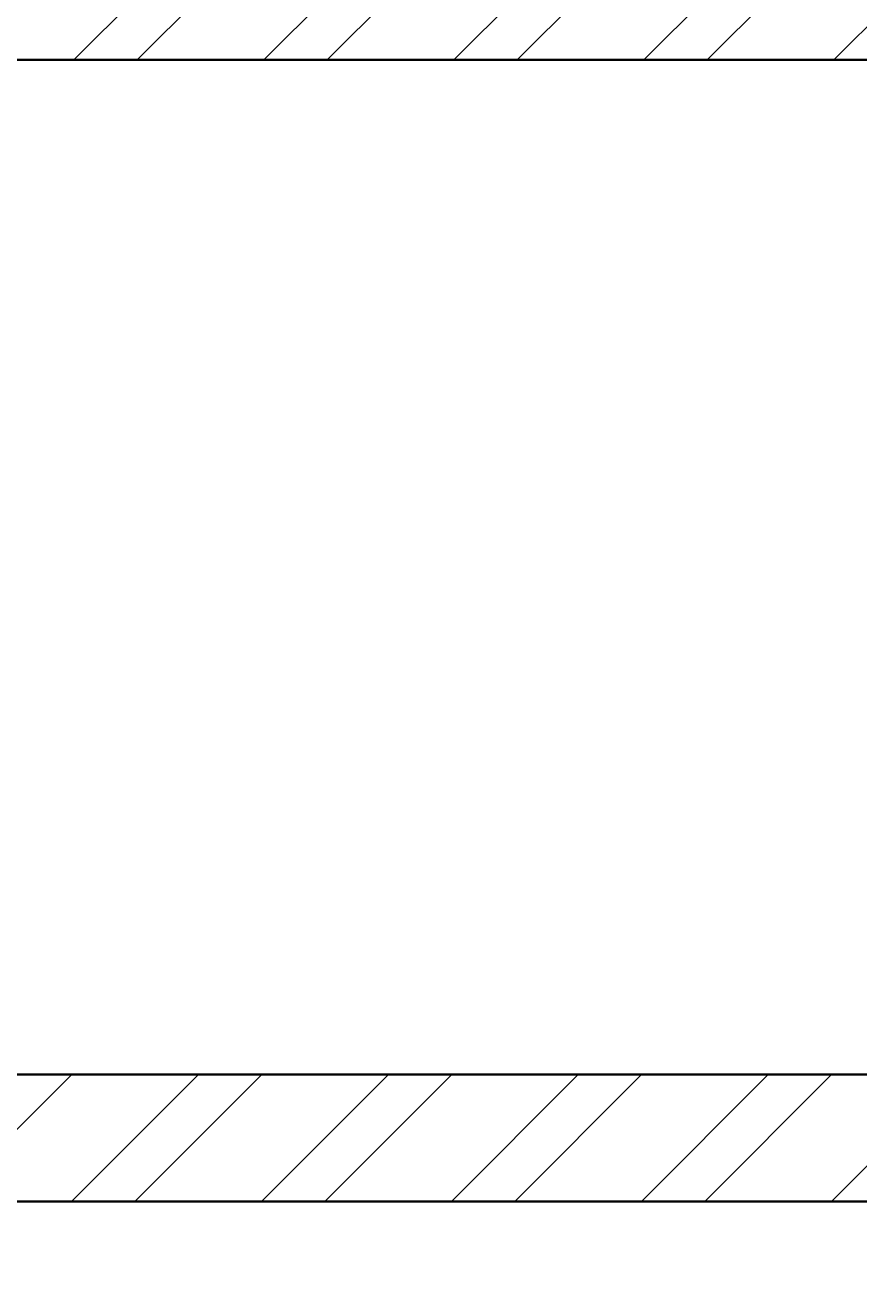
# Model space of a CAD drawing. Units: inches. Extents: x 2166 to 3588, y 1959 to 2628.
# Tile 5 of 13: x 3339 to 3398, y 2016 to 2105. Entities that reach past the tile are written whole.
import ezdxf

# ---------------------------------------------------------------- set-up
doc = ezdxf.new("R2010")
doc.units = ezdxf.units.IN
for name, color, linetype, lineweight in [('A-ANNO-DIMS', 2, 'Continuous', 18), ('A-WALL-PATT', 20, 'Continuous', 13), ('WALL', 40, 'Continuous', 35)]:
    doc.layers.add(name, color=color, linetype=linetype, lineweight=lineweight)
doc.styles.get("Standard").update_dxf_attribs({"font": 'arial.ttf'})
doc.dimstyles.get("Standard").update_dxf_attribs({"dimtxt": 0.18, "dimasz": 0.18, "dimexe": 0.18, "dimexo": 0.0625, "dimgap": 0.09, "dimtad": 0, "dimtih": 1, "dimtoh": 1, "dimdec": 4, "dimzin": 0, "dimdsep": 46, "dimtxsty": 'Standard', "dimcen": 0.09, "dimadec": 0, "dimazin": 0, "dimtfac": 1, "dimtdec": 4, "dimtofl": 0, "dimtmove": 0, "dimatfit": 3, "dimfxl": 1, "dimtolj": 1, "dimtzin": 0, "dimarcsym": 0})

# ---------------------------------------------------------------- blocks, each defined once
blk = doc.blocks.new('*D50')
at = {"layer": 'A-ANNO-DIMS', "color": 0, "lineweight": -2, "transparency": 16777216}
for p, q in [((3236.471, 2030.916), (3236.471, 1997.049)), ((3428.471, 2030.916), (3428.471, 1997.049)), ((3236.651, 1997.229), (3332.191, 1997.229)), ((3428.291, 1997.229), (3332.75, 1997.229))]:
    blk.add_line(p, q, dxfattribs=at)
at = {"layer": 'A-ANNO-DIMS', "color": 0, "transparency": 16777216}
for points in [[(3236.651, 1997.259), (3236.651, 1997.199), (3236.471, 1997.229)], [(3428.291, 1997.259), (3428.291, 1997.199), (3428.471, 1997.229)]]:
    blk.add_solid(points, dxfattribs=at)
at = {"layer": 'Defpoints', "color": 0, "transparency": 16777216}
for p in [(3236.471, 2030.979), (3428.471, 2030.979), (3428.471, 1997.229)]:
    blk.add_point(p, dxfattribs=at)
at = {"layer": 'A-ANNO-DIMS', "color": 0, "transparency": 16777216, "insert": (3332.471, 1997.229), "char_height": 0.18, "attachment_point": 5}
blk.add_mtext('\\A1;192', dxfattribs=at)

msp = doc.modelspace()

# ---------------------------------------------------------------- hatches: boundary and pattern name
at = {"layer": 'A-WALL-PATT'}
h = msp.add_hatch(dxfattribs=at)
h.set_pattern_fill('ANSI32', color=256)
h.paths.add_polyline_path([(3563.471, 2429.979), (3227.471, 2429.979), (3227.471, 2021.979), (3563.471, 2021.979)])
h.paths.add_polyline_path([(3236.471, 2420.979), (3554.471, 2420.979), (3554.471, 2111.979), (3236.471, 2111.979)], flags=16)
h.paths.add_polyline_path([(3236.471, 2102.979), (3554.471, 2102.979), (3554.471, 2030.979), (3236.471, 2030.979)], flags=16)
h.paths.add_polyline_path([(3518.471, 2085.283), (3518.471, 2067.979), (3458.471, 2067.979), (3458.471, 2085.283)], flags=0)
h.paths.add_polyline_path([(3434.656, 2082.283), (3442.194, 2082.283), (3442.194, 2087.514), (3434.656, 2087.514)], flags=8)
h.paths.add_polyline_path([(3522.671, 2094.512), (3521.752, 2052.984), (3545.541, 2052.457), (3546.46, 2093.986)], flags=8)

# ---------------------------------------------------------------- linework, layer by layer
at = {"layer": 'WALL'}
msp.add_line((3554.471, 2102.979), (3236.471, 2102.979), dxfattribs=at)
msp.add_lwpolyline([(3227.471, 2429.979), (3563.471, 2429.979), (3563.471, 2021.979), (3227.471, 2021.979)], close=True, dxfattribs=at)
msp.add_lwpolyline([(3554.471, 2102.979), (3554.471, 2030.979), (3236.471, 2030.979), (3236.471, 2102.979)], dxfattribs=at)

# ---------------------------------------------------------------- dimensions: what is measured, and where the dimension line sits
at = {"layer": 'A-ANNO-DIMS'}
dim = msp.add_linear_dim(base=(3428.471, 1997.229), p1=(3236.471, 2030.979), p2=(3428.471, 2030.979), dimstyle='Standard', override={"dimdec": 0, "dimlfac": 1, "dimrnd": 0, "dimzin": 0, "dimdsep": 46, "dimlunit": 2}, dxfattribs=at)
dim.commit()
dim.dimension.update_dxf_attribs({"geometry": '*D50', "text_midpoint": (3332.471, 1997.229)})

doc.saveas('drawing.dxf')
